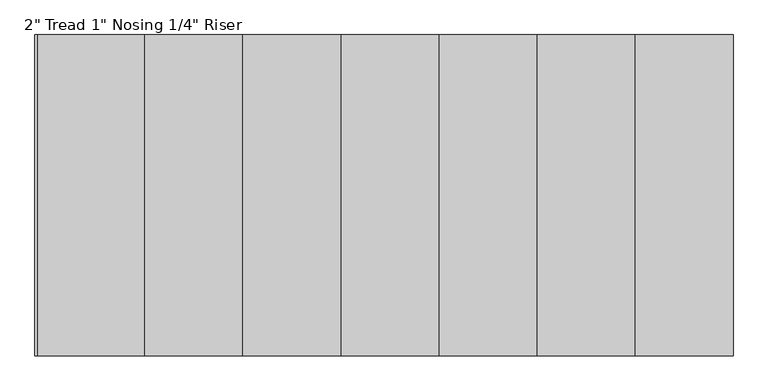
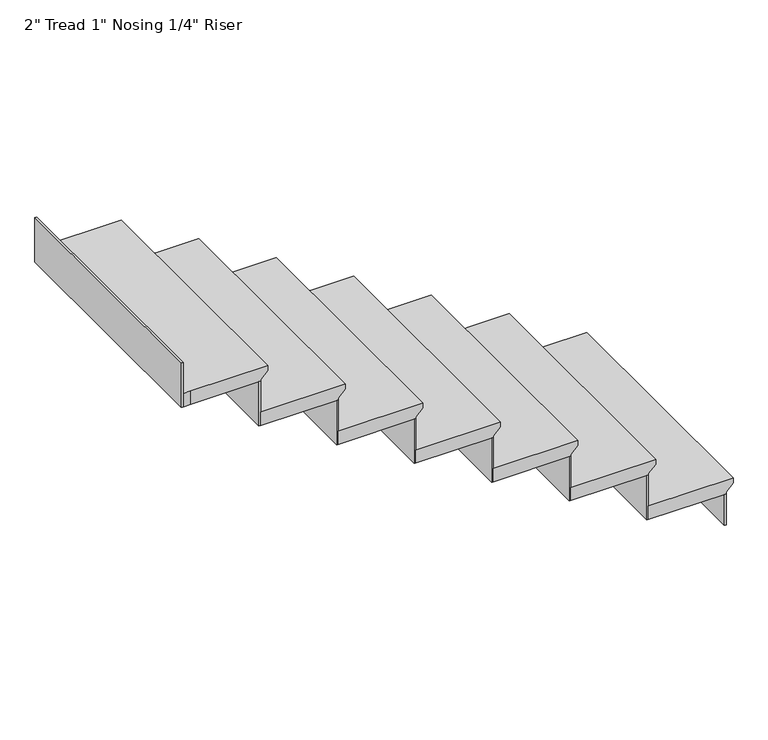
"""IFC4 building model written with IfcOpenShell, lengths in millimetres: stair flight geometry."""

from ifc_helpers import new_model, si_unit, origin, place, context, project, spatial, faceted_brep, source, transform, mapped, element, save


def stair_flight_92885a51(model_context):
    return source(origin(), model_context, "Body", "Brep", [
        faceted_brep([(-11420.6750862, 7015.0620171, 150.2833333), (-11420.6750862, 7015.0620171, 169.3333333), (-11420.6750862, 6100.6620171, 169.3333333), (-11420.6750862, 6100.6620171, 150.2833333), (-11446.0750862, 7015.0620171, 124.8833333), (-11446.0750862, 6100.6620171, 124.8833333), (-11725.4750862, 7015.0620171, 169.3333333), (-11725.4750862, 6100.6620171, 169.3333333), (-11446.0750862, 6100.6620171, 118.5333333), (-11725.4750862, 6100.6620171, 118.5333333), (-11725.4750862, 7015.0620171, 118.5333333), (-11446.0750862, 7015.0620171, 118.5333333)], [[[0, 1, 2, 3]], [[4, 0, 3, 5]], [[2, 1, 6, 7]], [[8, 9, 10, 11]], [[2, 7, 9, 8, 5, 3]], [[8, 11, 4, 5]], [[6, 1, 0, 4, 11, 10]], [[7, 6, 10, 9]]]),
        faceted_brep([(-11446.0750862, 7015.0620171, 118.5333333), (-11446.0750862, 7015.0620171, 0.0), (-11452.4250862, 7015.0620171, 0.0), (-11452.4250862, 7015.0620171, 118.5333333), (-11446.0750862, 6100.6620171, 118.5333333), (-11452.4250862, 6100.6620171, 118.5333333), (-11452.4250862, 6100.6620171, 0.0), (-11446.0750862, 6100.6620171, 0.0)], [[[0, 1, 2, 3]], [[4, 5, 6, 7]], [[1, 0, 4, 7]], [[2, 1, 7, 6]], [[3, 2, 6, 5]], [[0, 3, 5, 4]]]),
        faceted_brep([(-13401.8750862, 7015.0620171, 1303.8666667), (-13401.8750862, 7015.0620171, 1134.5333333), (-13408.2250862, 7015.0620171, 1134.5333333), (-13408.2250862, 7015.0620171, 1303.8666667), (-13401.8750862, 6100.6620171, 1303.8666667), (-13408.2250862, 6100.6620171, 1303.8666667), (-13408.2250862, 6100.6620171, 1134.5333333), (-13401.8750862, 6100.6620171, 1134.5333333)], [[[0, 1, 2, 3]], [[4, 5, 6, 7]], [[1, 0, 4, 7]], [[2, 1, 7, 6]], [[3, 2, 6, 5]], [[0, 3, 5, 4]]]),
        faceted_brep([(-11725.4750862, 7015.0620171, 287.8666667), (-11725.4750862, 7015.0620171, 118.5333333), (-11731.8250862, 7015.0620171, 118.5333333), (-11731.8250862, 7015.0620171, 287.8666667), (-11725.4750862, 6100.6620171, 287.8666667), (-11731.8250862, 6100.6620171, 287.8666667), (-11731.8250862, 6100.6620171, 118.5333333), (-11725.4750862, 6100.6620171, 118.5333333)], [[[0, 1, 2, 3]], [[4, 5, 6, 7]], [[1, 0, 4, 7]], [[2, 1, 7, 6]], [[3, 2, 6, 5]], [[0, 3, 5, 4]]]),
        faceted_brep([(-11700.0750862, 6100.6620171, 338.6666667), (-11700.0750862, 7015.0620171, 338.6666667), (-12004.8750862, 7015.0620171, 338.6666667), (-12004.8750862, 6100.6620171, 338.6666667), (-11725.4750862, 6100.6620171, 287.8666667), (-12004.8750862, 6100.6620171, 287.8666667), (-12004.8750862, 7015.0620171, 287.8666667), (-11725.4750862, 7015.0620171, 287.8666667), (-11725.4750862, 6100.6620171, 294.2166667), (-11700.0750862, 6100.6620171, 319.6166667), (-11725.4750862, 7015.0620171, 294.2166667), (-11700.0750862, 7015.0620171, 319.6166667)], [[[0, 1, 2, 3]], [[4, 5, 6, 7]], [[0, 3, 5, 4, 8, 9]], [[4, 7, 10, 8]], [[2, 1, 11, 10, 7, 6]], [[3, 2, 6, 5]], [[11, 1, 0, 9]], [[10, 11, 9, 8]]]),
        faceted_brep([(-12004.8750862, 7015.0620171, 457.2), (-12004.8750862, 7015.0620171, 287.8666667), (-12011.2250862, 7015.0620171, 287.8666667), (-12011.2250862, 7015.0620171, 457.2), (-12004.8750862, 6100.6620171, 457.2), (-12011.2250862, 6100.6620171, 457.2), (-12011.2250862, 6100.6620171, 287.8666667), (-12004.8750862, 6100.6620171, 287.8666667)], [[[0, 1, 2, 3]], [[4, 5, 6, 7]], [[1, 0, 4, 7]], [[2, 1, 7, 6]], [[3, 2, 6, 5]], [[0, 3, 5, 4]]]),
        faceted_brep([(-11979.4750862, 6100.6620171, 508.0), (-11979.4750862, 7015.0620171, 508.0), (-12284.2750862, 7015.0620171, 508.0), (-12284.2750862, 6100.6620171, 508.0), (-12004.8750862, 6100.6620171, 457.2), (-12284.2750862, 6100.6620171, 457.2), (-12284.2750862, 7015.0620171, 457.2), (-12004.8750862, 7015.0620171, 457.2), (-12004.8750862, 6100.6620171, 463.55), (-11979.4750862, 6100.6620171, 488.95), (-12004.8750862, 7015.0620171, 463.55), (-11979.4750862, 7015.0620171, 488.95)], [[[0, 1, 2, 3]], [[4, 5, 6, 7]], [[0, 3, 5, 4, 8, 9]], [[4, 7, 10, 8]], [[2, 1, 11, 10, 7, 6]], [[3, 2, 6, 5]], [[11, 1, 0, 9]], [[10, 11, 9, 8]]]),
        faceted_brep([(-12284.2750862, 7015.0620171, 626.5333333), (-12284.2750862, 7015.0620171, 457.2), (-12290.6250862, 7015.0620171, 457.2), (-12290.6250862, 7015.0620171, 626.5333333), (-12284.2750862, 6100.6620171, 626.5333333), (-12290.6250862, 6100.6620171, 626.5333333), (-12290.6250862, 6100.6620171, 457.2), (-12284.2750862, 6100.6620171, 457.2)], [[[0, 1, 2, 3]], [[4, 5, 6, 7]], [[1, 0, 4, 7]], [[2, 1, 7, 6]], [[3, 2, 6, 5]], [[0, 3, 5, 4]]]),
        faceted_brep([(-12258.8750862, 6100.6620171, 677.3333333), (-12258.8750862, 7015.0620171, 677.3333333), (-12563.6750862, 7015.0620171, 677.3333333), (-12563.6750862, 6100.6620171, 677.3333333), (-12284.2750862, 6100.6620171, 626.5333333), (-12563.6750862, 6100.6620171, 626.5333333), (-12563.6750862, 7015.0620171, 626.5333333), (-12284.2750862, 7015.0620171, 626.5333333), (-12284.2750862, 6100.6620171, 632.8833333), (-12258.8750862, 6100.6620171, 658.2833333), (-12284.2750862, 7015.0620171, 632.8833333), (-12258.8750862, 7015.0620171, 658.2833333)], [[[0, 1, 2, 3]], [[4, 5, 6, 7]], [[0, 3, 5, 4, 8, 9]], [[4, 7, 10, 8]], [[2, 1, 11, 10, 7, 6]], [[3, 2, 6, 5]], [[11, 1, 0, 9]], [[10, 11, 9, 8]]]),
        faceted_brep([(-12563.6750862, 7015.0620171, 795.8666667), (-12563.6750862, 7015.0620171, 626.5333333), (-12570.0250862, 7015.0620171, 626.5333333), (-12570.0250862, 7015.0620171, 795.8666667), (-12563.6750862, 6100.6620171, 795.8666667), (-12570.0250862, 6100.6620171, 795.8666667), (-12570.0250862, 6100.6620171, 626.5333333), (-12563.6750862, 6100.6620171, 626.5333333)], [[[0, 1, 2, 3]], [[4, 5, 6, 7]], [[1, 0, 4, 7]], [[2, 1, 7, 6]], [[3, 2, 6, 5]], [[0, 3, 5, 4]]]),
        faceted_brep([(-12538.2750862, 6100.6620171, 846.6666667), (-12538.2750862, 7015.0620171, 846.6666667), (-12843.0750862, 7015.0620171, 846.6666667), (-12843.0750862, 6100.6620171, 846.6666667), (-12563.6750862, 6100.6620171, 795.8666667), (-12843.0750862, 6100.6620171, 795.8666667), (-12843.0750862, 7015.0620171, 795.8666667), (-12563.6750862, 7015.0620171, 795.8666667), (-12563.6750862, 6100.6620171, 802.2166667), (-12538.2750862, 6100.6620171, 827.6166667), (-12563.6750862, 7015.0620171, 802.2166667), (-12538.2750862, 7015.0620171, 827.6166667)], [[[0, 1, 2, 3]], [[4, 5, 6, 7]], [[0, 3, 5, 4, 8, 9]], [[4, 7, 10, 8]], [[2, 1, 11, 10, 7, 6]], [[3, 2, 6, 5]], [[11, 1, 0, 9]], [[10, 11, 9, 8]]]),
        faceted_brep([(-12843.0750862, 7015.0620171, 965.2), (-12843.0750862, 7015.0620171, 795.8666667), (-12849.4250862, 7015.0620171, 795.8666667), (-12849.4250862, 7015.0620171, 965.2), (-12843.0750862, 6100.6620171, 965.2), (-12849.4250862, 6100.6620171, 965.2), (-12849.4250862, 6100.6620171, 795.8666667), (-12843.0750862, 6100.6620171, 795.8666667)], [[[0, 1, 2, 3]], [[4, 5, 6, 7]], [[1, 0, 4, 7]], [[2, 1, 7, 6]], [[3, 2, 6, 5]], [[0, 3, 5, 4]]]),
        faceted_brep([(-12817.6750862, 6100.6620171, 1016.0), (-12817.6750862, 7015.0620171, 1016.0), (-13122.4750862, 7015.0620171, 1016.0), (-13122.4750862, 6100.6620171, 1016.0), (-12843.0750862, 6100.6620171, 965.2), (-13122.4750862, 6100.6620171, 965.2), (-13122.4750862, 7015.0620171, 965.2), (-12843.0750862, 7015.0620171, 965.2), (-12843.0750862, 6100.6620171, 971.55), (-12817.6750862, 6100.6620171, 996.95), (-12843.0750862, 7015.0620171, 971.55), (-12817.6750862, 7015.0620171, 996.95)], [[[0, 1, 2, 3]], [[4, 5, 6, 7]], [[0, 3, 5, 4, 8, 9]], [[4, 7, 10, 8]], [[2, 1, 11, 10, 7, 6]], [[3, 2, 6, 5]], [[11, 1, 0, 9]], [[10, 11, 9, 8]]]),
        faceted_brep([(-13122.4750862, 7015.0620171, 1134.5333333), (-13122.4750862, 7015.0620171, 965.2), (-13128.8250862, 7015.0620171, 965.2), (-13128.8250862, 7015.0620171, 1134.5333333), (-13122.4750862, 6100.6620171, 1134.5333333), (-13128.8250862, 6100.6620171, 1134.5333333), (-13128.8250862, 6100.6620171, 965.2), (-13122.4750862, 6100.6620171, 965.2)], [[[0, 1, 2, 3]], [[4, 5, 6, 7]], [[1, 0, 4, 7]], [[2, 1, 7, 6]], [[3, 2, 6, 5]], [[0, 3, 5, 4]]]),
        faceted_brep([(-13401.8750862, 6100.6620171, 1185.3333333), (-13376.4750862, 6100.6620171, 1185.3333333), (-13097.0750862, 6100.6620171, 1185.3333333), (-13097.0750862, 7015.0620171, 1185.3333333), (-13401.8750862, 7015.0620171, 1185.3333333), (-13376.4750862, 6100.6620171, 1134.5333333), (-13401.8750862, 6100.6620171, 1134.5333333), (-13401.8750862, 7015.0620171, 1134.5333333), (-13122.4750862, 7015.0620171, 1134.5333333), (-13122.4750862, 6100.6620171, 1134.5333333), (-13122.4750862, 6100.6620171, 1140.8833333), (-13097.0750862, 6100.6620171, 1166.2833333), (-13122.4750862, 7015.0620171, 1140.8833333), (-13097.0750862, 7015.0620171, 1166.2833333)], [[[0, 1, 2, 3, 4]], [[5, 6, 7, 8, 9]], [[1, 0, 6, 5]], [[2, 1, 5, 9, 10, 11]], [[9, 8, 12, 10]], [[4, 3, 13, 12, 8, 7]], [[0, 4, 7, 6]], [[13, 3, 2, 11]], [[12, 13, 11, 10]]]),
    ])


if __name__ == "__main__":
    model = new_model("IFC4")
    model_context = context("Model", 3, world=origin())
    ifc_project = project(units=[si_unit("LENGTHUNIT", "METRE", prefix="MILLI")], contexts=[model_context])
    site = spatial("IfcSite", under=ifc_project)
    building = spatial("IfcBuilding", under=site)
    placement = place(None, origin())
    stair_flight_shape = stair_flight_92885a51(model_context)
    element("IfcStairFlight", 1, ObjectType="2\" Tread 1\" Nosing 1/4\" Riser", at=placement, inside=building, context=model_context, shape_type="MappedRepresentation", body=[
        mapped(stair_flight_shape, transform((0.0, 0.0, 0.0), x_axis=(1.0, 0.0, 0.0), y_axis=(0.0, 1.0, 0.0), z_axis=(0.0, 0.0, 1.0))),
    ])
    save(model, "model.ifc")
